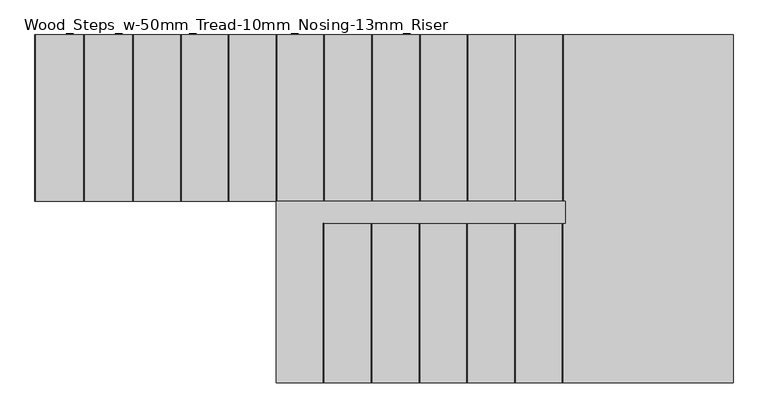
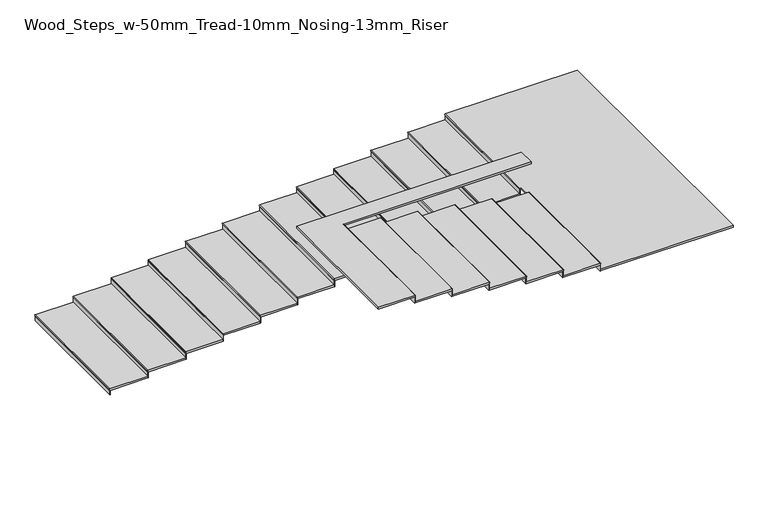
"""IFC4 building model written with IfcOpenShell, lengths in millimetres: stair flight geometry, Wood_Steps_w-50mm_Tread-10mm_Nosing-13mm_Riser."""

from ifc_helpers import new_model, si_unit, frame, origin, place, context, project, spatial, circle_curve, faceted_brep, source, transform, mapped, element, save
from ifc_brep_helpers import plane_surface, cylinder_surface, advanced_brep


def wood_steps_w_50mm_tread_10mm_nosing_13mm_riser_e98e060e(model_context):
    return source(origin(), model_context, "Body", "SolidModel", [
        advanced_brep(
        [(-49046.7440401, 412.2005214, 146.6666667), (-49046.7440401, 412.2005214, 166.6666667), (-49046.7440401, 3859.4375818, 166.6666667), (-49046.7440401, 3859.4375818, 146.6666667), (-48030.7440401, 3859.4375818, 166.6666667), (-48030.7440401, 412.2005214, 166.6666667), (-49046.7440401, 3859.4375818, 116.6666667), (-48030.7440401, 3859.4375818, 116.6666667), (-48030.7440401, 412.2005214, 116.6666667), (-49046.7440401, 412.2005214, 116.6666667)],
        [
            (0, 1, circle_curve(frame((-49046.7440401, 412.2005214, 156.6666667), z_axis=(0.0, 1.0, 0.0), x_axis=(1.0, 0.0, 0.0)), 10.0)),
            (1, 2),
            (2, 3, circle_curve(frame((-49046.7440401, 3859.4375818, 156.6666667), z_axis=(0.0, -1.0, 0.0), x_axis=(1.0, 0.0, 0.0)), 10.0)),
            (3, 0),
            (4, 2),
            (1, 5),
            (5, 4),
            (6, 7),
            (7, 8),
            (8, 9),
            (9, 6),
            (4, 7),
            (6, 3),
            (9, 0),
            (8, 5),
        ],
        [
            cylinder_surface(frame((-49046.7440401, 412.2005214, 156.6666667), z_axis=(0.0, -1.0, 0.0), x_axis=(1.0, 0.0, 0.0)), 10.0),
            plane_surface(frame((-49056.7440401, 3859.4375818, 166.6666667), z_axis=(0.0, 0.0, 1.0), x_axis=(-1.0, 0.0, 0.0))),
            plane_surface(frame((-49056.7440401, 3859.4375818, 116.6666667), z_axis=(0.0, 0.0, -1.0), x_axis=(1.0, 0.0, 0.0))),
            plane_surface(frame((-48030.7440401, 3859.4375818, 166.6666667), z_axis=(0.0, 1.0, 0.0), x_axis=(0.0, 0.0, -1.0))),
            plane_surface(frame((-49046.7440401, 3859.4375818, 166.6666667), z_axis=(-1.0, 0.0, 0.0), x_axis=(0.0, 0.0, -1.0))),
            plane_surface(frame((-49046.7440401, 412.2005214, 166.6666667), z_axis=(0.0, -1.0, 0.0), x_axis=(0.0, 0.0, -1.0))),
            plane_surface(frame((-48030.7440401, 412.2005214, 166.6666667), z_axis=(1.0, 0.0, 0.0), x_axis=(0.0, 0.0, -1.0))),
        ],
        [
            (0, [[1, 2, 3, 4]]),
            (1, [[5, -2, 6, 7]]),
            (2, [[8, 9, 10, 11]]),
            (3, [[-5, 12, -8, 13, -3]]),
            (4, [[-11, 14, -4, -13]]),
            (5, [[-6, -1, -14, -10, 15]]),
            (6, [[-7, -15, -9, -12]]),
        ],
    ),
        faceted_brep([(-49046.7440401, 412.2005214, 116.6666667), (-49046.7440401, 412.2005214, 0.0), (-49034.2440401, 412.2005214, 0.0), (-49034.2440401, 412.2005214, 116.6666667), (-49046.7440401, 3859.4375818, 116.6666667), (-49034.2440401, 3859.4375818, 116.6666667), (-49034.2440401, 3859.4375818, 0.0), (-49046.7440401, 3859.4375818, 0.0)], [[[0, 1, 2, 3]], [[4, 5, 6, 7]], [[1, 0, 4, 7]], [[2, 1, 7, 6]], [[3, 2, 6, 5]], [[0, 3, 5, 4]]]),
        faceted_brep([(-48030.7440401, 412.2005214, 283.3333333), (-48030.7440401, 412.2005214, 116.6666667), (-48018.2440401, 412.2005214, 116.6666667), (-48018.2440401, 412.2005214, 283.3333333), (-48030.7440401, 3859.4375818, 283.3333333), (-48018.2440401, 3859.4375818, 283.3333333), (-48018.2440401, 3859.4375818, 116.6666667), (-48030.7440401, 3859.4375818, 116.6666667)], [[[0, 1, 2, 3]], [[4, 5, 6, 7]], [[1, 0, 4, 7]], [[2, 1, 7, 6]], [[3, 2, 6, 5]], [[0, 3, 5, 4]]]),
        advanced_brep(
        [(-47014.7440401, 3859.4375818, 333.3333333), (-48030.7440401, 3859.4375818, 333.3333333), (-48030.7440401, 412.2005214, 333.3333333), (-47014.7440401, 412.2005214, 333.3333333), (-48030.7440401, 3859.4375818, 283.3333333), (-47014.7440401, 3859.4375818, 283.3333333), (-47014.7440401, 412.2005214, 283.3333333), (-48030.7440401, 412.2005214, 283.3333333), (-48030.7440401, 3859.4375818, 313.3333333), (-48030.7440401, 412.2005214, 313.3333333)],
        [
            (0, 1),
            (1, 2),
            (2, 3),
            (3, 0),
            (4, 5),
            (5, 6),
            (6, 7),
            (7, 4),
            (0, 5),
            (4, 8),
            (8, 1, circle_curve(frame((-48030.7440401, 3859.4375818, 323.3333333), z_axis=(0.0, 1.0, 0.0), x_axis=(1.0, 0.0, 0.0)), 10.0)),
            (7, 9),
            (9, 8),
            (2, 9, circle_curve(frame((-48030.7440401, 412.2005214, 323.3333333), z_axis=(0.0, -1.0, 0.0), x_axis=(1.0, 0.0, 0.0)), 10.0)),
            (6, 3),
        ],
        [
            plane_surface(frame((-49056.7440401, 3859.4375818, 333.3333333), z_axis=(0.0, 0.0, 1.0), x_axis=(-1.0, 0.0, 0.0))),
            plane_surface(frame((-49056.7440401, 3859.4375818, 283.3333333), z_axis=(0.0, 0.0, -1.0), x_axis=(1.0, 0.0, 0.0))),
            plane_surface(frame((-47014.7440401, 3859.4375818, 333.3333333), z_axis=(0.0, 1.0, 0.0), x_axis=(0.0, 0.0, -1.0))),
            plane_surface(frame((-48030.7440401, 3859.4375818, 333.3333333), z_axis=(-1.0, 0.0, 0.0), x_axis=(0.0, 0.0, -1.0))),
            plane_surface(frame((-48030.7440401, 412.2005214, 333.3333333), z_axis=(0.0, -1.0, 0.0), x_axis=(0.0, 0.0, -1.0))),
            plane_surface(frame((-47014.7440401, 412.2005214, 333.3333333), z_axis=(1.0, 0.0, 0.0), x_axis=(0.0, 0.0, -1.0))),
            cylinder_surface(frame((-48030.7440401, 412.2005214, 323.3333333), z_axis=(0.0, -1.0, 0.0), x_axis=(1.0, 0.0, 0.0)), 10.0),
        ],
        [
            (0, [[1, 2, 3, 4]]),
            (1, [[5, 6, 7, 8]]),
            (2, [[-1, 9, -5, 10, 11]]),
            (3, [[-8, 12, 13, -10]]),
            (4, [[-3, 14, -12, -7, 15]]),
            (5, [[-4, -15, -6, -9]]),
            (6, [[-14, -2, -11, -13]]),
        ],
    ),
        faceted_brep([(-47014.7440401, 412.2005214, 450.0), (-47014.7440401, 412.2005214, 283.3333333), (-47002.2440401, 412.2005214, 283.3333333), (-47002.2440401, 412.2005214, 450.0), (-47014.7440401, 3859.4375818, 450.0), (-47002.2440401, 3859.4375818, 450.0), (-47002.2440401, 3859.4375818, 283.3333333), (-47014.7440401, 3859.4375818, 283.3333333)], [[[0, 1, 2, 3]], [[4, 5, 6, 7]], [[1, 0, 4, 7]], [[2, 1, 7, 6]], [[3, 2, 6, 5]], [[0, 3, 5, 4]]]),
        advanced_brep(
        [(-46024.1440401, 3859.4375818, 500.0), (-47014.7440401, 3859.4375818, 500.0), (-47014.7440401, 412.2005214, 500.0), (-46024.1440401, 412.2005214, 500.0), (-47014.7440401, 3859.4375818, 450.0), (-46024.1440401, 3859.4375818, 450.0), (-46024.1440401, 412.2005214, 450.0), (-47014.7440401, 412.2005214, 450.0), (-47014.7440401, 3859.4375818, 480.0), (-47014.7440401, 412.2005214, 480.0)],
        [
            (0, 1),
            (1, 2),
            (2, 3),
            (3, 0),
            (4, 5),
            (5, 6),
            (6, 7),
            (7, 4),
            (0, 5),
            (4, 8),
            (8, 1, circle_curve(frame((-47014.7440401, 3859.4375818, 490.0), z_axis=(0.0, 1.0, 0.0), x_axis=(1.0, 0.0, 0.0)), 10.0)),
            (7, 9),
            (9, 8),
            (2, 9, circle_curve(frame((-47014.7440401, 412.2005214, 490.0), z_axis=(0.0, -1.0, 0.0), x_axis=(1.0, 0.0, 0.0)), 10.0)),
            (6, 3),
        ],
        [
            plane_surface(frame((-49056.7440401, 3859.4375818, 500.0), z_axis=(0.0, 0.0, 1.0), x_axis=(-1.0, 0.0, 0.0))),
            plane_surface(frame((-49056.7440401, 3859.4375818, 450.0), z_axis=(0.0, 0.0, -1.0), x_axis=(1.0, 0.0, 0.0))),
            plane_surface(frame((-46024.1440401, 3859.4375818, 500.0), z_axis=(0.0, 1.0, 0.0), x_axis=(0.0, 0.0, -1.0))),
            plane_surface(frame((-47014.7440401, 3859.4375818, 500.0), z_axis=(-1.0, 0.0, 0.0), x_axis=(0.0, 0.0, -1.0))),
            plane_surface(frame((-47014.7440401, 412.2005214, 500.0), z_axis=(0.0, -1.0, 0.0), x_axis=(0.0, 0.0, -1.0))),
            plane_surface(frame((-46024.1440401, 412.2005214, 500.0), z_axis=(1.0, 0.0, 0.0), x_axis=(0.0, 0.0, -1.0))),
            cylinder_surface(frame((-47014.7440401, 412.2005214, 490.0), z_axis=(0.0, -1.0, 0.0), x_axis=(1.0, 0.0, 0.0)), 10.0),
        ],
        [
            (0, [[1, 2, 3, 4]]),
            (1, [[5, 6, 7, 8]]),
            (2, [[-1, 9, -5, 10, 11]]),
            (3, [[-8, 12, 13, -10]]),
            (4, [[-3, 14, -12, -7, 15]]),
            (5, [[-4, -15, -6, -9]]),
            (6, [[-14, -2, -11, -13]]),
        ],
    ),
        faceted_brep([(-46024.1440401, 412.2005214, 616.6666667), (-46024.1440401, 412.2005214, 450.0), (-46011.6440401, 412.2005214, 450.0), (-46011.6440401, 412.2005214, 616.6666667), (-46024.1440401, 3859.4375818, 616.6666667), (-46011.6440401, 3859.4375818, 616.6666667), (-46011.6440401, 3859.4375818, 450.0), (-46024.1440401, 3859.4375818, 450.0)], [[[0, 1, 2, 3]], [[4, 5, 6, 7]], [[1, 0, 4, 7]], [[2, 1, 7, 6]], [[3, 2, 6, 5]], [[0, 3, 5, 4]]]),
        advanced_brep(
        [(-45033.5440401, 3859.4375818, 666.6666667), (-46024.1440401, 3859.4375818, 666.6666667), (-46024.1440401, 412.2005214, 666.6666667), (-45033.5440401, 412.2005214, 666.6666667), (-46024.1440401, 3859.4375818, 616.6666667), (-45033.5440401, 3859.4375818, 616.6666667), (-45033.5440401, 412.2005214, 616.6666667), (-46024.1440401, 412.2005214, 616.6666667), (-46024.1440401, 3859.4375818, 646.6666667), (-46024.1440401, 412.2005214, 646.6666667)],
        [
            (0, 1),
            (1, 2),
            (2, 3),
            (3, 0),
            (4, 5),
            (5, 6),
            (6, 7),
            (7, 4),
            (0, 5),
            (4, 8),
            (8, 1, circle_curve(frame((-46024.1440401, 3859.4375818, 656.6666667), z_axis=(0.0, 1.0, 0.0), x_axis=(1.0, 0.0, 0.0)), 10.0)),
            (7, 9),
            (9, 8),
            (2, 9, circle_curve(frame((-46024.1440401, 412.2005214, 656.6666667), z_axis=(0.0, -1.0, 0.0), x_axis=(1.0, 0.0, 0.0)), 10.0)),
            (6, 3),
        ],
        [
            plane_surface(frame((-48066.1440401, 3859.4375818, 666.6666667), z_axis=(0.0, 0.0, 1.0), x_axis=(-1.0, 0.0, 0.0))),
            plane_surface(frame((-48066.1440401, 3859.4375818, 616.6666667), z_axis=(0.0, 0.0, -1.0), x_axis=(1.0, 0.0, 0.0))),
            plane_surface(frame((-45033.5440401, 3859.4375818, 666.6666667), z_axis=(0.0, 1.0, 0.0), x_axis=(0.0, 0.0, -1.0))),
            plane_surface(frame((-46024.1440401, 3859.4375818, 666.6666667), z_axis=(-1.0, 0.0, 0.0), x_axis=(0.0, 0.0, -1.0))),
            plane_surface(frame((-46024.1440401, 412.2005214, 666.6666667), z_axis=(0.0, -1.0, 0.0), x_axis=(0.0, 0.0, -1.0))),
            plane_surface(frame((-45033.5440401, 412.2005214, 666.6666667), z_axis=(1.0, 0.0, 0.0), x_axis=(0.0, 0.0, -1.0))),
            cylinder_surface(frame((-46024.1440401, 412.2005214, 656.6666667), z_axis=(0.0, -1.0, 0.0), x_axis=(1.0, 0.0, 0.0)), 10.0),
        ],
        [
            (0, [[1, 2, 3, 4]]),
            (1, [[5, 6, 7, 8]]),
            (2, [[-1, 9, -5, 10, 11]]),
            (3, [[-8, 12, 13, -10]]),
            (4, [[-3, 14, -12, -7, 15]]),
            (5, [[-4, -15, -6, -9]]),
            (6, [[-14, -2, -11, -13]]),
        ],
    ),
        faceted_brep([(-45033.5440401, 412.2005214, 783.3333333), (-45033.5440401, 412.2005214, 616.6666667), (-45021.0440401, 412.2005214, 616.6666667), (-45021.0440401, 412.2005214, 783.3333333), (-45033.5440401, 3859.4375818, 783.3333333), (-45021.0440401, 3859.4375818, 783.3333333), (-45021.0440401, 3859.4375818, 616.6666667), (-45033.5440401, 3859.4375818, 616.6666667)], [[[0, 1, 2, 3]], [[4, 5, 6, 7]], [[1, 0, 4, 7]], [[2, 1, 7, 6]], [[3, 2, 6, 5]], [[0, 3, 5, 4]]]),
        advanced_brep(
        [(-44042.9440401, 3859.4375818, 833.3333333), (-45033.5440401, 3859.4375818, 833.3333333), (-45033.5440401, 412.2005214, 833.3333333), (-44042.9440401, 412.2005214, 833.3333333), (-45033.5440401, 3859.4375818, 783.3333333), (-44042.9440401, 3859.4375818, 783.3333333), (-44042.9440401, 412.2005214, 783.3333333), (-45033.5440401, 412.2005214, 783.3333333), (-45033.5440401, 3859.4375818, 813.3333333), (-45033.5440401, 412.2005214, 813.3333333)],
        [
            (0, 1),
            (1, 2),
            (2, 3),
            (3, 0),
            (4, 5),
            (5, 6),
            (6, 7),
            (7, 4),
            (0, 5),
            (4, 8),
            (8, 1, circle_curve(frame((-45033.5440401, 3859.4375818, 823.3333333), z_axis=(0.0, 1.0, 0.0), x_axis=(1.0, 0.0, 0.0)), 10.0)),
            (7, 9),
            (9, 8),
            (2, 9, circle_curve(frame((-45033.5440401, 412.2005214, 823.3333333), z_axis=(0.0, -1.0, 0.0), x_axis=(1.0, 0.0, 0.0)), 10.0)),
            (6, 3),
        ],
        [
            plane_surface(frame((-47075.5440401, 3859.4375818, 833.3333333), z_axis=(0.0, 0.0, 1.0), x_axis=(-1.0, 0.0, 0.0))),
            plane_surface(frame((-47075.5440401, 3859.4375818, 783.3333333), z_axis=(0.0, 0.0, -1.0), x_axis=(1.0, 0.0, 0.0))),
            plane_surface(frame((-44042.9440401, 3859.4375818, 833.3333333), z_axis=(0.0, 1.0, 0.0), x_axis=(0.0, 0.0, -1.0))),
            plane_surface(frame((-45033.5440401, 3859.4375818, 833.3333333), z_axis=(-1.0, 0.0, 0.0), x_axis=(0.0, 0.0, -1.0))),
            plane_surface(frame((-45033.5440401, 412.2005214, 833.3333333), z_axis=(0.0, -1.0, 0.0), x_axis=(0.0, 0.0, -1.0))),
            plane_surface(frame((-44042.9440401, 412.2005214, 833.3333333), z_axis=(1.0, 0.0, 0.0), x_axis=(0.0, 0.0, -1.0))),
            cylinder_surface(frame((-45033.5440401, 412.2005214, 823.3333333), z_axis=(0.0, -1.0, 0.0), x_axis=(1.0, 0.0, 0.0)), 10.0),
        ],
        [
            (0, [[1, 2, 3, 4]]),
            (1, [[5, 6, 7, 8]]),
            (2, [[-1, 9, -5, 10, 11]]),
            (3, [[-8, 12, 13, -10]]),
            (4, [[-3, 14, -12, -7, 15]]),
            (5, [[-4, -15, -6, -9]]),
            (6, [[-14, -2, -11, -13]]),
        ],
    ),
        faceted_brep([(-44042.9440401, 412.2005214, 950.0), (-44042.9440401, 412.2005214, 783.3333333), (-44030.4440401, 412.2005214, 783.3333333), (-44030.4440401, 412.2005214, 950.0), (-44042.9440401, 3859.4375818, 950.0), (-44030.4440401, 3859.4375818, 950.0), (-44030.4440401, 3859.4375818, 783.3333333), (-44042.9440401, 3859.4375818, 783.3333333)], [[[0, 1, 2, 3]], [[4, 5, 6, 7]], [[1, 0, 4, 7]], [[2, 1, 7, 6]], [[3, 2, 6, 5]], [[0, 3, 5, 4]]]),
        advanced_brep(
        [(-43052.3440401, 3859.4375818, 1000.0), (-44042.9440401, 3859.4375818, 1000.0), (-44042.9440401, 412.2005214, 1000.0), (-43052.3440401, 412.2005214, 1000.0), (-44042.9440401, 3859.4375818, 950.0), (-43052.3440401, 3859.4375818, 950.0), (-43052.3440401, 412.2005214, 950.0), (-44042.9440401, 412.2005214, 950.0), (-44042.9440401, 3859.4375818, 980.0), (-44042.9440401, 412.2005214, 980.0)],
        [
            (0, 1),
            (1, 2),
            (2, 3),
            (3, 0),
            (4, 5),
            (5, 6),
            (6, 7),
            (7, 4),
            (0, 5),
            (4, 8),
            (8, 1, circle_curve(frame((-44042.9440401, 3859.4375818, 990.0), z_axis=(0.0, 1.0, 0.0), x_axis=(1.0, 0.0, 0.0)), 10.0)),
            (7, 9),
            (9, 8),
            (2, 9, circle_curve(frame((-44042.9440401, 412.2005214, 990.0), z_axis=(0.0, -1.0, 0.0), x_axis=(1.0, 0.0, 0.0)), 10.0)),
            (6, 3),
        ],
        [
            plane_surface(frame((-46084.9440401, 3859.4375818, 1000.0), z_axis=(0.0, 0.0, 1.0), x_axis=(-1.0, 0.0, 0.0))),
            plane_surface(frame((-46084.9440401, 3859.4375818, 950.0), z_axis=(0.0, 0.0, -1.0), x_axis=(1.0, 0.0, 0.0))),
            plane_surface(frame((-43052.3440401, 3859.4375818, 1000.0), z_axis=(0.0, 1.0, 0.0), x_axis=(0.0, 0.0, -1.0))),
            plane_surface(frame((-44042.9440401, 3859.4375818, 1000.0), z_axis=(-1.0, 0.0, 0.0), x_axis=(0.0, 0.0, -1.0))),
            plane_surface(frame((-44042.9440401, 412.2005214, 1000.0), z_axis=(0.0, -1.0, 0.0), x_axis=(0.0, 0.0, -1.0))),
            plane_surface(frame((-43052.3440401, 412.2005214, 1000.0), z_axis=(1.0, 0.0, 0.0), x_axis=(0.0, 0.0, -1.0))),
            cylinder_surface(frame((-44042.9440401, 412.2005214, 990.0), z_axis=(0.0, -1.0, 0.0), x_axis=(1.0, 0.0, 0.0)), 10.0),
        ],
        [
            (0, [[1, 2, 3, 4]]),
            (1, [[5, 6, 7, 8]]),
            (2, [[-1, 9, -5, 10, 11]]),
            (3, [[-8, 12, 13, -10]]),
            (4, [[-3, 14, -12, -7, 15]]),
            (5, [[-4, -15, -6, -9]]),
            (6, [[-14, -2, -11, -13]]),
        ],
    ),
        faceted_brep([(-43052.3440401, 412.2005214, 1116.6666667), (-43052.3440401, 412.2005214, 950.0), (-43039.8440401, 412.2005214, 950.0), (-43039.8440401, 412.2005214, 1116.6666667), (-43052.3440401, 3859.4375818, 1116.6666667), (-43039.8440401, 3859.4375818, 1116.6666667), (-43039.8440401, 3859.4375818, 950.0), (-43052.3440401, 3859.4375818, 950.0)], [[[0, 1, 2, 3]], [[4, 5, 6, 7]], [[1, 0, 4, 7]], [[2, 1, 7, 6]], [[3, 2, 6, 5]], [[0, 3, 5, 4]]]),
        advanced_brep(
        [(-42061.7440401, 3859.4375818, 1166.6666667), (-43052.3440401, 3859.4375818, 1166.6666667), (-43052.3440401, 412.2005214, 1166.6666667), (-42061.7440401, 412.2005214, 1166.6666667), (-43052.3440401, 3859.4375818, 1116.6666667), (-42061.7440401, 3859.4375818, 1116.6666667), (-42061.7440401, 412.2005214, 1116.6666667), (-43052.3440401, 412.2005214, 1116.6666667), (-43052.3440401, 3859.4375818, 1146.6666667), (-43052.3440401, 412.2005214, 1146.6666667)],
        [
            (0, 1),
            (1, 2),
            (2, 3),
            (3, 0),
            (4, 5),
            (5, 6),
            (6, 7),
            (7, 4),
            (0, 5),
            (4, 8),
            (8, 1, circle_curve(frame((-43052.3440401, 3859.4375818, 1156.6666667), z_axis=(0.0, 1.0, 0.0), x_axis=(1.0, 0.0, 0.0)), 10.0)),
            (7, 9),
            (9, 8),
            (2, 9, circle_curve(frame((-43052.3440401, 412.2005214, 1156.6666667), z_axis=(0.0, -1.0, 0.0), x_axis=(1.0, 0.0, 0.0)), 10.0)),
            (6, 3),
        ],
        [
            plane_surface(frame((-45094.3440401, 3859.4375818, 1166.6666667), z_axis=(0.0, 0.0, 1.0), x_axis=(-1.0, 0.0, 0.0))),
            plane_surface(frame((-45094.3440401, 3859.4375818, 1116.6666667), z_axis=(0.0, 0.0, -1.0), x_axis=(1.0, 0.0, 0.0))),
            plane_surface(frame((-42061.7440401, 3859.4375818, 1166.6666667), z_axis=(0.0, 1.0, 0.0), x_axis=(0.0, 0.0, -1.0))),
            plane_surface(frame((-43052.3440401, 3859.4375818, 1166.6666667), z_axis=(-1.0, 0.0, 0.0), x_axis=(0.0, 0.0, -1.0))),
            plane_surface(frame((-43052.3440401, 412.2005214, 1166.6666667), z_axis=(0.0, -1.0, 0.0), x_axis=(0.0, 0.0, -1.0))),
            plane_surface(frame((-42061.7440401, 412.2005214, 1166.6666667), z_axis=(1.0, 0.0, 0.0), x_axis=(0.0, 0.0, -1.0))),
            cylinder_surface(frame((-43052.3440401, 412.2005214, 1156.6666667), z_axis=(0.0, -1.0, 0.0), x_axis=(1.0, 0.0, 0.0)), 10.0),
        ],
        [
            (0, [[1, 2, 3, 4]]),
            (1, [[5, 6, 7, 8]]),
            (2, [[-1, 9, -5, 10, 11]]),
            (3, [[-8, 12, 13, -10]]),
            (4, [[-3, 14, -12, -7, 15]]),
            (5, [[-4, -15, -6, -9]]),
            (6, [[-14, -2, -11, -13]]),
        ],
    ),
        faceted_brep([(-42061.7440401, 412.2005214, 1283.3333333), (-42061.7440401, 412.2005214, 1116.6666667), (-42049.2440401, 412.2005214, 1116.6666667), (-42049.2440401, 412.2005214, 1283.3333333), (-42061.7440401, 3859.4375818, 1283.3333333), (-42049.2440401, 3859.4375818, 1283.3333333), (-42049.2440401, 3859.4375818, 1116.6666667), (-42061.7440401, 3859.4375818, 1116.6666667)], [[[0, 1, 2, 3]], [[4, 5, 6, 7]], [[1, 0, 4, 7]], [[2, 1, 7, 6]], [[3, 2, 6, 5]], [[0, 3, 5, 4]]]),
        advanced_brep(
        [(-41071.1440401, 3859.4375818, 1333.3333333), (-42061.7440401, 3859.4375818, 1333.3333333), (-42061.7440401, 412.2005214, 1333.3333333), (-41071.1440401, 412.2005214, 1333.3333333), (-42061.7440401, 3859.4375818, 1283.3333333), (-41071.1440401, 3859.4375818, 1283.3333333), (-41071.1440401, 412.2005214, 1283.3333333), (-42061.7440401, 412.2005214, 1283.3333333), (-42061.7440401, 3859.4375818, 1313.3333333), (-42061.7440401, 412.2005214, 1313.3333333)],
        [
            (0, 1),
            (1, 2),
            (2, 3),
            (3, 0),
            (4, 5),
            (5, 6),
            (6, 7),
            (7, 4),
            (0, 5),
            (4, 8),
            (8, 1, circle_curve(frame((-42061.7440401, 3859.4375818, 1323.3333333), z_axis=(0.0, 1.0, 0.0), x_axis=(1.0, 0.0, 0.0)), 10.0)),
            (7, 9),
            (9, 8),
            (2, 9, circle_curve(frame((-42061.7440401, 412.2005214, 1323.3333333), z_axis=(0.0, -1.0, 0.0), x_axis=(1.0, 0.0, 0.0)), 10.0)),
            (6, 3),
        ],
        [
            plane_surface(frame((-44103.7440401, 3859.4375818, 1333.3333333), z_axis=(0.0, 0.0, 1.0), x_axis=(-1.0, 0.0, 0.0))),
            plane_surface(frame((-44103.7440401, 3859.4375818, 1283.3333333), z_axis=(0.0, 0.0, -1.0), x_axis=(1.0, 0.0, 0.0))),
            plane_surface(frame((-41071.1440401, 3859.4375818, 1333.3333333), z_axis=(0.0, 1.0, 0.0), x_axis=(0.0, 0.0, -1.0))),
            plane_surface(frame((-42061.7440401, 3859.4375818, 1333.3333333), z_axis=(-1.0, 0.0, 0.0), x_axis=(0.0, 0.0, -1.0))),
            plane_surface(frame((-42061.7440401, 412.2005214, 1333.3333333), z_axis=(0.0, -1.0, 0.0), x_axis=(0.0, 0.0, -1.0))),
            plane_surface(frame((-41071.1440401, 412.2005214, 1333.3333333), z_axis=(1.0, 0.0, 0.0), x_axis=(0.0, 0.0, -1.0))),
            cylinder_surface(frame((-42061.7440401, 412.2005214, 1323.3333333), z_axis=(0.0, -1.0, 0.0), x_axis=(1.0, 0.0, 0.0)), 10.0),
        ],
        [
            (0, [[1, 2, 3, 4]]),
            (1, [[5, 6, 7, 8]]),
            (2, [[-1, 9, -5, 10, 11]]),
            (3, [[-8, 12, 13, -10]]),
            (4, [[-3, 14, -12, -7, 15]]),
            (5, [[-4, -15, -6, -9]]),
            (6, [[-14, -2, -11, -13]]),
        ],
    ),
        faceted_brep([(-41071.1440401, 412.2005214, 1450.0), (-41071.1440401, 412.2005214, 1283.3333333), (-41058.6440401, 412.2005214, 1283.3333333), (-41058.6440401, 412.2005214, 1450.0), (-41071.1440401, 3859.4375818, 1450.0), (-41058.6440401, 3859.4375818, 1450.0), (-41058.6440401, 3859.4375818, 1283.3333333), (-41071.1440401, 3859.4375818, 1283.3333333)], [[[0, 1, 2, 3]], [[4, 5, 6, 7]], [[1, 0, 4, 7]], [[2, 1, 7, 6]], [[3, 2, 6, 5]], [[0, 3, 5, 4]]]),
        advanced_brep(
        [(-40080.5440401, 3859.4375818, 1500.0), (-41071.1440401, 3859.4375818, 1500.0), (-41071.1440401, 412.2005214, 1500.0), (-40080.5440401, 412.2005214, 1500.0), (-41071.1440401, 3859.4375818, 1450.0), (-40080.5440401, 3859.4375818, 1450.0), (-40080.5440401, 412.2005214, 1450.0), (-41071.1440401, 412.2005214, 1450.0), (-41071.1440401, 3859.4375818, 1480.0), (-41071.1440401, 412.2005214, 1480.0)],
        [
            (0, 1),
            (1, 2),
            (2, 3),
            (3, 0),
            (4, 5),
            (5, 6),
            (6, 7),
            (7, 4),
            (0, 5),
            (4, 8),
            (8, 1, circle_curve(frame((-41071.1440401, 3859.4375818, 1490.0), z_axis=(0.0, 1.0, 0.0), x_axis=(1.0, 0.0, 0.0)), 10.0)),
            (7, 9),
            (9, 8),
            (2, 9, circle_curve(frame((-41071.1440401, 412.2005214, 1490.0), z_axis=(0.0, -1.0, 0.0), x_axis=(1.0, 0.0, 0.0)), 10.0)),
            (6, 3),
        ],
        [
            plane_surface(frame((-43113.1440401, 3859.4375818, 1500.0), z_axis=(0.0, 0.0, 1.0), x_axis=(-1.0, 0.0, 0.0))),
            plane_surface(frame((-43113.1440401, 3859.4375818, 1450.0), z_axis=(0.0, 0.0, -1.0), x_axis=(1.0, 0.0, 0.0))),
            plane_surface(frame((-40080.5440401, 3859.4375818, 1500.0), z_axis=(0.0, 1.0, 0.0), x_axis=(0.0, 0.0, -1.0))),
            plane_surface(frame((-41071.1440401, 3859.4375818, 1500.0), z_axis=(-1.0, 0.0, 0.0), x_axis=(0.0, 0.0, -1.0))),
            plane_surface(frame((-41071.1440401, 412.2005214, 1500.0), z_axis=(0.0, -1.0, 0.0), x_axis=(0.0, 0.0, -1.0))),
            plane_surface(frame((-40080.5440401, 412.2005214, 1500.0), z_axis=(1.0, 0.0, 0.0), x_axis=(0.0, 0.0, -1.0))),
            cylinder_surface(frame((-41071.1440401, 412.2005214, 1490.0), z_axis=(0.0, -1.0, 0.0), x_axis=(1.0, 0.0, 0.0)), 10.0),
        ],
        [
            (0, [[1, 2, 3, 4]]),
            (1, [[5, 6, 7, 8]]),
            (2, [[-1, 9, -5, 10, 11]]),
            (3, [[-8, 12, 13, -10]]),
            (4, [[-3, 14, -12, -7, 15]]),
            (5, [[-4, -15, -6, -9]]),
            (6, [[-14, -2, -11, -13]]),
        ],
    ),
        faceted_brep([(-40080.5440401, 412.2005214, 1616.6666667), (-40080.5440401, 412.2005214, 1450.0), (-40068.0440401, 412.2005214, 1450.0), (-40068.0440401, 412.2005214, 1616.6666667), (-40080.5440401, 3859.4375818, 1616.6666667), (-40068.0440401, 3859.4375818, 1616.6666667), (-40068.0440401, 3859.4375818, 1450.0), (-40080.5440401, 3859.4375818, 1450.0)], [[[0, 1, 2, 3]], [[4, 5, 6, 7]], [[1, 0, 4, 7]], [[2, 1, 7, 6]], [[3, 2, 6, 5]], [[0, 3, 5, 4]]]),
        advanced_brep(
        [(-39089.9440401, 3859.4375818, 1666.6666667), (-40080.5440401, 3859.4375818, 1666.6666667), (-40080.5440401, 412.2005214, 1666.6666667), (-39089.9440401, 412.2005214, 1666.6666667), (-40080.5440401, 3859.4375818, 1616.6666667), (-39089.9440401, 3859.4375818, 1616.6666667), (-39089.9440401, 412.2005214, 1616.6666667), (-40080.5440401, 412.2005214, 1616.6666667), (-40080.5440401, 3859.4375818, 1646.6666667), (-40080.5440401, 412.2005214, 1646.6666667)],
        [
            (0, 1),
            (1, 2),
            (2, 3),
            (3, 0),
            (4, 5),
            (5, 6),
            (6, 7),
            (7, 4),
            (0, 5),
            (4, 8),
            (8, 1, circle_curve(frame((-40080.5440401, 3859.4375818, 1656.6666667), z_axis=(0.0, 1.0, 0.0), x_axis=(1.0, 0.0, 0.0)), 10.0)),
            (7, 9),
            (9, 8),
            (2, 9, circle_curve(frame((-40080.5440401, 412.2005214, 1656.6666667), z_axis=(0.0, -1.0, 0.0), x_axis=(1.0, 0.0, 0.0)), 10.0)),
            (6, 3),
        ],
        [
            plane_surface(frame((-42122.5440401, 3859.4375818, 1666.6666667), z_axis=(0.0, 0.0, 1.0), x_axis=(-1.0, 0.0, 0.0))),
            plane_surface(frame((-42122.5440401, 3859.4375818, 1616.6666667), z_axis=(0.0, 0.0, -1.0), x_axis=(1.0, 0.0, 0.0))),
            plane_surface(frame((-39089.9440401, 3859.4375818, 1666.6666667), z_axis=(0.0, 1.0, 0.0), x_axis=(0.0, 0.0, -1.0))),
            plane_surface(frame((-40080.5440401, 3859.4375818, 1666.6666667), z_axis=(-1.0, 0.0, 0.0), x_axis=(0.0, 0.0, -1.0))),
            plane_surface(frame((-40080.5440401, 412.2005214, 1666.6666667), z_axis=(0.0, -1.0, 0.0), x_axis=(0.0, 0.0, -1.0))),
            plane_surface(frame((-39089.9440401, 412.2005214, 1666.6666667), z_axis=(1.0, 0.0, 0.0), x_axis=(0.0, 0.0, -1.0))),
            cylinder_surface(frame((-40080.5440401, 412.2005214, 1656.6666667), z_axis=(0.0, -1.0, 0.0), x_axis=(1.0, 0.0, 0.0)), 10.0),
        ],
        [
            (0, [[1, 2, 3, 4]]),
            (1, [[5, 6, 7, 8]]),
            (2, [[-1, 9, -5, 10, 11]]),
            (3, [[-8, 12, 13, -10]]),
            (4, [[-3, 14, -12, -7, 15]]),
            (5, [[-4, -15, -6, -9]]),
            (6, [[-14, -2, -11, -13]]),
        ],
    ),
        faceted_brep([(-39089.9440401, 412.2005214, 1783.3333333), (-39089.9440401, 412.2005214, 1616.6666667), (-39077.4440401, 412.2005214, 1616.6666667), (-39077.4440401, 412.2005214, 1783.3333333), (-39089.9440401, 3859.4375818, 1783.3333333), (-39077.4440401, 3859.4375818, 1783.3333333), (-39077.4440401, 3859.4375818, 1616.6666667), (-39089.9440401, 3859.4375818, 1616.6666667)], [[[0, 1, 2, 3]], [[4, 5, 6, 7]], [[1, 0, 4, 7]], [[2, 1, 7, 6]], [[3, 2, 6, 5]], [[0, 3, 5, 4]]]),
        advanced_brep(
        [(-38099.3440401, 3859.4375818, 1833.3333333), (-39089.9440401, 3859.4375818, 1833.3333333), (-39089.9440401, 412.2005214, 1833.3333333), (-38099.3440401, 412.2005214, 1833.3333333), (-39089.9440401, 3859.4375818, 1783.3333333), (-38099.3440401, 3859.4375818, 1783.3333333), (-38099.3440401, 412.2005214, 1783.3333333), (-39089.9440401, 412.2005214, 1783.3333333), (-39089.9440401, 3859.4375818, 1813.3333333), (-39089.9440401, 412.2005214, 1813.3333333)],
        [
            (0, 1),
            (1, 2),
            (2, 3),
            (3, 0),
            (4, 5),
            (5, 6),
            (6, 7),
            (7, 4),
            (0, 5),
            (4, 8),
            (8, 1, circle_curve(frame((-39089.9440401, 3859.4375818, 1823.3333333), z_axis=(0.0, 1.0, 0.0), x_axis=(1.0, 0.0, 0.0)), 10.0)),
            (7, 9),
            (9, 8),
            (2, 9, circle_curve(frame((-39089.9440401, 412.2005214, 1823.3333333), z_axis=(0.0, -1.0, 0.0), x_axis=(1.0, 0.0, 0.0)), 10.0)),
            (6, 3),
        ],
        [
            plane_surface(frame((-41131.9440401, 3859.4375818, 1833.3333333), z_axis=(0.0, 0.0, 1.0), x_axis=(-1.0, 0.0, 0.0))),
            plane_surface(frame((-41131.9440401, 3859.4375818, 1783.3333333), z_axis=(0.0, 0.0, -1.0), x_axis=(1.0, 0.0, 0.0))),
            plane_surface(frame((-38099.3440401, 3859.4375818, 1833.3333333), z_axis=(0.0, 1.0, 0.0), x_axis=(0.0, 0.0, -1.0))),
            plane_surface(frame((-39089.9440401, 3859.4375818, 1833.3333333), z_axis=(-1.0, 0.0, 0.0), x_axis=(0.0, 0.0, -1.0))),
            plane_surface(frame((-39089.9440401, 412.2005214, 1833.3333333), z_axis=(0.0, -1.0, 0.0), x_axis=(0.0, 0.0, -1.0))),
            plane_surface(frame((-38099.3440401, 412.2005214, 1833.3333333), z_axis=(1.0, 0.0, 0.0), x_axis=(0.0, 0.0, -1.0))),
            cylinder_surface(frame((-39089.9440401, 412.2005214, 1823.3333333), z_axis=(0.0, -1.0, 0.0), x_axis=(1.0, 0.0, 0.0)), 10.0),
        ],
        [
            (0, [[1, 2, 3, 4]]),
            (1, [[5, 6, 7, 8]]),
            (2, [[-1, 9, -5, 10, 11]]),
            (3, [[-8, 12, 13, -10]]),
            (4, [[-3, 14, -12, -7, 15]]),
            (5, [[-4, -15, -6, -9]]),
            (6, [[-14, -2, -11, -13]]),
        ],
    ),
        faceted_brep([(-38099.3440401, 412.2005214, 1950.0), (-38099.3440401, 412.2005214, 1783.3333333), (-38086.8440401, 412.2005214, 1783.3333333), (-38086.8440401, 412.2005214, 1950.0), (-38099.3440401, 3859.4375818, 1950.0), (-38086.8440401, 3859.4375818, 1950.0), (-38086.8440401, 3859.4375818, 1783.3333333), (-38099.3440401, 3859.4375818, 1783.3333333)], [[[0, 1, 2, 3]], [[4, 5, 6, 7]], [[1, 0, 4, 7]], [[2, 1, 7, 6]], [[3, 2, 6, 5]], [[0, 3, 5, 4]]]),
        advanced_brep(
        [(-38119.3440401, -3354.1624182, 2000.0), (-34578.7440401, -3354.1624182, 2000.0), (-34578.7440401, 3859.4375818, 2000.0), (-38099.3440401, 3859.4375818, 2000.0), (-38099.3440401, 412.2005214, 2000.0), (-38062.0088218, 412.2005214, 2000.0), (-38062.0088218, -44.9994786, 2000.0), (-38119.3440401, -44.9994786, 2000.0), (-34578.7440401, -3354.1624182, 1950.0), (-38119.3440401, -3354.1624182, 1950.0), (-38119.3440401, -44.9994786, 1950.0), (-38062.0088218, -44.9994786, 1950.0), (-38062.0088218, 412.2005214, 1950.0), (-38099.3440401, 412.2005214, 1950.0), (-38099.3440401, 3859.4375818, 1950.0), (-34578.7440401, 3859.4375818, 1950.0), (-38099.3440401, 3859.4375818, 1980.0), (-38099.3440401, 412.2005214, 1980.0)],
        [
            (0, 1),
            (1, 2),
            (2, 3),
            (3, 4),
            (4, 5),
            (5, 6),
            (6, 7),
            (7, 0),
            (8, 9),
            (9, 10),
            (10, 11),
            (11, 12),
            (12, 13),
            (13, 14),
            (14, 15),
            (15, 8),
            (0, 9),
            (8, 1),
            (15, 2),
            (14, 16),
            (16, 3, circle_curve(frame((-38099.3440401, 3859.4375818, 1990.0), z_axis=(0.0, 1.0, 0.0), x_axis=(1.0, 0.0, 0.0)), 10.0)),
            (13, 17),
            (17, 16),
            (4, 17, circle_curve(frame((-38099.3440401, 412.2005214, 1990.0), z_axis=(0.0, -1.0, 0.0), x_axis=(1.0, 0.0, 0.0)), 10.0)),
            (12, 5),
            (11, 6),
            (10, 7),
        ],
        [
            plane_surface(frame((-34578.7440401, -3354.1624182, 2000.0), z_axis=(0.0, 0.0, 1.0), x_axis=(1.0, 0.0, 0.0))),
            plane_surface(frame((-34578.7440401, -3354.1624182, 1950.0), z_axis=(0.0, 0.0, -1.0), x_axis=(-1.0, 0.0, 0.0))),
            plane_surface(frame((-38119.3440401, -3354.1624182, 2000.0), z_axis=(0.0, -1.0, 0.0), x_axis=(0.0, 0.0, -1.0))),
            plane_surface(frame((-34578.7440401, -3354.1624182, 2000.0), z_axis=(1.0, 0.0, 0.0), x_axis=(0.0, 0.0, -1.0))),
            plane_surface(frame((-34578.7440401, 3859.4375818, 2000.0), z_axis=(0.0, 1.0, 0.0), x_axis=(0.0, 0.0, -1.0))),
            plane_surface(frame((-38099.3440401, 3859.4375818, 2000.0), z_axis=(-1.0, 0.0, 0.0), x_axis=(0.0, 0.0, -1.0))),
            plane_surface(frame((-38099.3440401, 412.2005214, 2000.0), z_axis=(0.0, -1.0, 0.0), x_axis=(0.0, 0.0, -1.0))),
            plane_surface(frame((-38062.0088218, 412.2005214, 2000.0), z_axis=(-1.0, 0.0, 0.0), x_axis=(0.0, 0.0, -1.0))),
            plane_surface(frame((-38062.0088218, -44.9994786, 2000.0), z_axis=(0.0, 1.0, 0.0), x_axis=(0.0, 0.0, -1.0))),
            plane_surface(frame((-38119.3440401, -44.9994786, 2000.0), z_axis=(-1.0, 0.0, 0.0), x_axis=(0.0, 0.0, -1.0))),
            cylinder_surface(frame((-38099.3440401, 412.2005214, 1990.0), z_axis=(0.0, -1.0, 0.0), x_axis=(1.0, 0.0, 0.0)), 10.0),
        ],
        [
            (0, [[1, 2, 3, 4, 5, 6, 7, 8]]),
            (1, [[9, 10, 11, 12, 13, 14, 15, 16]]),
            (2, [[-1, 17, -9, 18]]),
            (3, [[-2, -18, -16, 19]]),
            (4, [[-3, -19, -15, 20, 21]]),
            (5, [[-14, 22, 23, -20]]),
            (6, [[-5, 24, -22, -13, 25]]),
            (7, [[-6, -25, -12, 26]]),
            (8, [[-7, -26, -11, 27]]),
            (9, [[-8, -27, -10, -17]]),
            (10, [[-24, -4, -21, -23]]),
        ],
    ),
        faceted_brep([(-38119.3440401, -44.9994786, 2116.6666667), (-38119.3440401, -44.9994786, 1950.0), (-38131.8440401, -44.9994786, 1950.0), (-38131.8440401, -44.9994786, 2116.6666667), (-38119.3440401, -3354.1624182, 2116.6666667), (-38131.8440401, -3354.1624182, 2116.6666667), (-38131.8440401, -3354.1624182, 1950.0), (-38119.3440401, -3354.1624182, 1950.0)], [[[0, 1, 2, 3]], [[4, 5, 6, 7]], [[1, 0, 4, 7]], [[2, 1, 7, 6]], [[3, 2, 6, 5]], [[0, 3, 5, 4]]]),
        advanced_brep(
        [(-39109.9440401, -3354.1624182, 2166.6666667), (-38119.3440401, -3354.1624182, 2166.6666667), (-38119.3440401, -44.9994786, 2166.6666667), (-39109.9440401, -44.9994786, 2166.6666667), (-38119.3440401, -3354.1624182, 2116.6666667), (-39109.9440401, -3354.1624182, 2116.6666667), (-39109.9440401, -44.9994786, 2116.6666667), (-38119.3440401, -44.9994786, 2116.6666667), (-38119.3440401, -3354.1624182, 2146.6666667), (-38119.3440401, -44.9994786, 2146.6666667)],
        [
            (0, 1),
            (1, 2),
            (2, 3),
            (3, 0),
            (4, 5),
            (5, 6),
            (6, 7),
            (7, 4),
            (0, 5),
            (4, 8),
            (8, 1, circle_curve(frame((-38119.3440401, -3354.1624182, 2156.6666667), z_axis=(0.0, -1.0, 0.0), x_axis=(-1.0, 0.0, 0.0)), 10.0)),
            (7, 9),
            (9, 8),
            (2, 9, circle_curve(frame((-38119.3440401, -44.9994786, 2156.6666667), z_axis=(0.0, 1.0, 0.0), x_axis=(-1.0, 0.0, 0.0)), 10.0)),
            (6, 3),
        ],
        [
            plane_surface(frame((-34578.7440401, -3354.1624182, 2166.6666667), z_axis=(0.0, 0.0, 1.0), x_axis=(1.0, 0.0, 0.0))),
            plane_surface(frame((-34578.7440401, -3354.1624182, 2116.6666667), z_axis=(0.0, 0.0, -1.0), x_axis=(-1.0, 0.0, 0.0))),
            plane_surface(frame((-39109.9440401, -3354.1624182, 2166.6666667), z_axis=(0.0, -1.0, 0.0), x_axis=(0.0, 0.0, -1.0))),
            plane_surface(frame((-38119.3440401, -3354.1624182, 2166.6666667), z_axis=(1.0, 0.0, 0.0), x_axis=(0.0, 0.0, -1.0))),
            plane_surface(frame((-38119.3440401, -44.9994786, 2166.6666667), z_axis=(0.0, 1.0, 0.0), x_axis=(0.0, 0.0, -1.0))),
            plane_surface(frame((-39109.9440401, -44.9994786, 2166.6666667), z_axis=(-1.0, 0.0, 0.0), x_axis=(0.0, 0.0, -1.0))),
            cylinder_surface(frame((-38119.3440401, -44.9994786, 2156.6666667), z_axis=(0.0, 1.0, 0.0), x_axis=(-1.0, 0.0, 0.0)), 10.0),
        ],
        [
            (0, [[1, 2, 3, 4]]),
            (1, [[5, 6, 7, 8]]),
            (2, [[-1, 9, -5, 10, 11]]),
            (3, [[-8, 12, 13, -10]]),
            (4, [[-3, 14, -12, -7, 15]]),
            (5, [[-4, -15, -6, -9]]),
            (6, [[-14, -2, -11, -13]]),
        ],
    ),
        faceted_brep([(-39109.9440401, -44.9994786, 2283.3333333), (-39109.9440401, -44.9994786, 2116.6666667), (-39122.4440401, -44.9994786, 2116.6666667), (-39122.4440401, -44.9994786, 2283.3333333), (-39109.9440401, -3354.1624182, 2283.3333333), (-39122.4440401, -3354.1624182, 2283.3333333), (-39122.4440401, -3354.1624182, 2116.6666667), (-39109.9440401, -3354.1624182, 2116.6666667)], [[[0, 1, 2, 3]], [[4, 5, 6, 7]], [[1, 0, 4, 7]], [[2, 1, 7, 6]], [[3, 2, 6, 5]], [[0, 3, 5, 4]]]),
        advanced_brep(
        [(-40100.5440401, -3354.1624182, 2333.3333333), (-39109.9440401, -3354.1624182, 2333.3333333), (-39109.9440401, -44.9994786, 2333.3333333), (-40100.5440401, -44.9994786, 2333.3333333), (-39109.9440401, -3354.1624182, 2283.3333333), (-40100.5440401, -3354.1624182, 2283.3333333), (-40100.5440401, -44.9994786, 2283.3333333), (-39109.9440401, -44.9994786, 2283.3333333), (-39109.9440401, -3354.1624182, 2313.3333333), (-39109.9440401, -44.9994786, 2313.3333333)],
        [
            (0, 1),
            (1, 2),
            (2, 3),
            (3, 0),
            (4, 5),
            (5, 6),
            (6, 7),
            (7, 4),
            (0, 5),
            (4, 8),
            (8, 1, circle_curve(frame((-39109.9440401, -3354.1624182, 2323.3333333), z_axis=(0.0, -1.0, 0.0), x_axis=(-1.0, 0.0, 0.0)), 10.0)),
            (7, 9),
            (9, 8),
            (2, 9, circle_curve(frame((-39109.9440401, -44.9994786, 2323.3333333), z_axis=(0.0, 1.0, 0.0), x_axis=(-1.0, 0.0, 0.0)), 10.0)),
            (6, 3),
        ],
        [
            plane_surface(frame((-35569.3440401, -3354.1624182, 2333.3333333), z_axis=(0.0, 0.0, 1.0), x_axis=(1.0, 0.0, 0.0))),
            plane_surface(frame((-35569.3440401, -3354.1624182, 2283.3333333), z_axis=(0.0, 0.0, -1.0), x_axis=(-1.0, 0.0, 0.0))),
            plane_surface(frame((-40100.5440401, -3354.1624182, 2333.3333333), z_axis=(0.0, -1.0, 0.0), x_axis=(0.0, 0.0, -1.0))),
            plane_surface(frame((-39109.9440401, -3354.1624182, 2333.3333333), z_axis=(1.0, 0.0, 0.0), x_axis=(0.0, 0.0, -1.0))),
            plane_surface(frame((-39109.9440401, -44.9994786, 2333.3333333), z_axis=(0.0, 1.0, 0.0), x_axis=(0.0, 0.0, -1.0))),
            plane_surface(frame((-40100.5440401, -44.9994786, 2333.3333333), z_axis=(-1.0, 0.0, 0.0), x_axis=(0.0, 0.0, -1.0))),
            cylinder_surface(frame((-39109.9440401, -44.9994786, 2323.3333333), z_axis=(0.0, 1.0, 0.0), x_axis=(-1.0, 0.0, 0.0)), 10.0),
        ],
        [
            (0, [[1, 2, 3, 4]]),
            (1, [[5, 6, 7, 8]]),
            (2, [[-1, 9, -5, 10, 11]]),
            (3, [[-8, 12, 13, -10]]),
            (4, [[-3, 14, -12, -7, 15]]),
            (5, [[-4, -15, -6, -9]]),
            (6, [[-14, -2, -11, -13]]),
        ],
    ),
        faceted_brep([(-40100.5440401, -44.9994786, 2450.0), (-40100.5440401, -44.9994786, 2283.3333333), (-40113.0440401, -44.9994786, 2283.3333333), (-40113.0440401, -44.9994786, 2450.0), (-40100.5440401, -3354.1624182, 2450.0), (-40113.0440401, -3354.1624182, 2450.0), (-40113.0440401, -3354.1624182, 2283.3333333), (-40100.5440401, -3354.1624182, 2283.3333333)], [[[0, 1, 2, 3]], [[4, 5, 6, 7]], [[1, 0, 4, 7]], [[2, 1, 7, 6]], [[3, 2, 6, 5]], [[0, 3, 5, 4]]]),
        advanced_brep(
        [(-41091.1440401, -3354.1624182, 2500.0), (-40100.5440401, -3354.1624182, 2500.0), (-40100.5440401, -44.9994786, 2500.0), (-41091.1440401, -44.9994786, 2500.0), (-40100.5440401, -3354.1624182, 2450.0), (-41091.1440401, -3354.1624182, 2450.0), (-41091.1440401, -44.9994786, 2450.0), (-40100.5440401, -44.9994786, 2450.0), (-40100.5440401, -3354.1624182, 2480.0), (-40100.5440401, -44.9994786, 2480.0)],
        [
            (0, 1),
            (1, 2),
            (2, 3),
            (3, 0),
            (4, 5),
            (5, 6),
            (6, 7),
            (7, 4),
            (0, 5),
            (4, 8),
            (8, 1, circle_curve(frame((-40100.5440401, -3354.1624182, 2490.0), z_axis=(0.0, -1.0, 0.0), x_axis=(-1.0, 0.0, 0.0)), 10.0)),
            (7, 9),
            (9, 8),
            (2, 9, circle_curve(frame((-40100.5440401, -44.9994786, 2490.0), z_axis=(0.0, 1.0, 0.0), x_axis=(-1.0, 0.0, 0.0)), 10.0)),
            (6, 3),
        ],
        [
            plane_surface(frame((-36559.9440401, -3354.1624182, 2500.0), z_axis=(0.0, 0.0, 1.0), x_axis=(1.0, 0.0, 0.0))),
            plane_surface(frame((-36559.9440401, -3354.1624182, 2450.0), z_axis=(0.0, 0.0, -1.0), x_axis=(-1.0, 0.0, 0.0))),
            plane_surface(frame((-41091.1440401, -3354.1624182, 2500.0), z_axis=(0.0, -1.0, 0.0), x_axis=(0.0, 0.0, -1.0))),
            plane_surface(frame((-40100.5440401, -3354.1624182, 2500.0), z_axis=(1.0, 0.0, 0.0), x_axis=(0.0, 0.0, -1.0))),
            plane_surface(frame((-40100.5440401, -44.9994786, 2500.0), z_axis=(0.0, 1.0, 0.0), x_axis=(0.0, 0.0, -1.0))),
            plane_surface(frame((-41091.1440401, -44.9994786, 2500.0), z_axis=(-1.0, 0.0, 0.0), x_axis=(0.0, 0.0, -1.0))),
            cylinder_surface(frame((-40100.5440401, -44.9994786, 2490.0), z_axis=(0.0, 1.0, 0.0), x_axis=(-1.0, 0.0, 0.0)), 10.0),
        ],
        [
            (0, [[1, 2, 3, 4]]),
            (1, [[5, 6, 7, 8]]),
            (2, [[-1, 9, -5, 10, 11]]),
            (3, [[-8, 12, 13, -10]]),
            (4, [[-3, 14, -12, -7, 15]]),
            (5, [[-4, -15, -6, -9]]),
            (6, [[-14, -2, -11, -13]]),
        ],
    ),
        faceted_brep([(-41091.1440401, -44.9994786, 2616.6666667), (-41091.1440401, -44.9994786, 2450.0), (-41103.6440401, -44.9994786, 2450.0), (-41103.6440401, -44.9994786, 2616.6666667), (-41091.1440401, -3354.1624182, 2616.6666667), (-41103.6440401, -3354.1624182, 2616.6666667), (-41103.6440401, -3354.1624182, 2450.0), (-41091.1440401, -3354.1624182, 2450.0)], [[[0, 1, 2, 3]], [[4, 5, 6, 7]], [[1, 0, 4, 7]], [[2, 1, 7, 6]], [[3, 2, 6, 5]], [[0, 3, 5, 4]]]),
        advanced_brep(
        [(-42081.7440401, -3354.1624182, 2666.6666667), (-41091.1440401, -3354.1624182, 2666.6666667), (-41091.1440401, -44.9994786, 2666.6666667), (-42081.7440401, -44.9994786, 2666.6666667), (-41091.1440401, -3354.1624182, 2616.6666667), (-42081.7440401, -3354.1624182, 2616.6666667), (-42081.7440401, -44.9994786, 2616.6666667), (-41091.1440401, -44.9994786, 2616.6666667), (-41091.1440401, -3354.1624182, 2646.6666667), (-41091.1440401, -44.9994786, 2646.6666667)],
        [
            (0, 1),
            (1, 2),
            (2, 3),
            (3, 0),
            (4, 5),
            (5, 6),
            (6, 7),
            (7, 4),
            (0, 5),
            (4, 8),
            (8, 1, circle_curve(frame((-41091.1440401, -3354.1624182, 2656.6666667), z_axis=(0.0, -1.0, 0.0), x_axis=(-1.0, 0.0, 0.0)), 10.0)),
            (7, 9),
            (9, 8),
            (2, 9, circle_curve(frame((-41091.1440401, -44.9994786, 2656.6666667), z_axis=(0.0, 1.0, 0.0), x_axis=(-1.0, 0.0, 0.0)), 10.0)),
            (6, 3),
        ],
        [
            plane_surface(frame((-37550.5440401, -3354.1624182, 2666.6666667), z_axis=(0.0, 0.0, 1.0), x_axis=(1.0, 0.0, 0.0))),
            plane_surface(frame((-37550.5440401, -3354.1624182, 2616.6666667), z_axis=(0.0, 0.0, -1.0), x_axis=(-1.0, 0.0, 0.0))),
            plane_surface(frame((-42081.7440401, -3354.1624182, 2666.6666667), z_axis=(0.0, -1.0, 0.0), x_axis=(0.0, 0.0, -1.0))),
            plane_surface(frame((-41091.1440401, -3354.1624182, 2666.6666667), z_axis=(1.0, 0.0, 0.0), x_axis=(0.0, 0.0, -1.0))),
            plane_surface(frame((-41091.1440401, -44.9994786, 2666.6666667), z_axis=(0.0, 1.0, 0.0), x_axis=(0.0, 0.0, -1.0))),
            plane_surface(frame((-42081.7440401, -44.9994786, 2666.6666667), z_axis=(-1.0, 0.0, 0.0), x_axis=(0.0, 0.0, -1.0))),
            cylinder_surface(frame((-41091.1440401, -44.9994786, 2656.6666667), z_axis=(0.0, 1.0, 0.0), x_axis=(-1.0, 0.0, 0.0)), 10.0),
        ],
        [
            (0, [[1, 2, 3, 4]]),
            (1, [[5, 6, 7, 8]]),
            (2, [[-1, 9, -5, 10, 11]]),
            (3, [[-8, 12, 13, -10]]),
            (4, [[-3, 14, -12, -7, 15]]),
            (5, [[-4, -15, -6, -9]]),
            (6, [[-14, -2, -11, -13]]),
        ],
    ),
        faceted_brep([(-42081.7440401, -44.9994786, 2783.3333333), (-42081.7440401, -44.9994786, 2616.6666667), (-42094.2440401, -44.9994786, 2616.6666667), (-42094.2440401, -44.9994786, 2783.3333333), (-42081.7440401, -3354.1624182, 2783.3333333), (-42094.2440401, -3354.1624182, 2783.3333333), (-42094.2440401, -3354.1624182, 2616.6666667), (-42081.7440401, -3354.1624182, 2616.6666667)], [[[0, 1, 2, 3]], [[4, 5, 6, 7]], [[1, 0, 4, 7]], [[2, 1, 7, 6]], [[3, 2, 6, 5]], [[0, 3, 5, 4]]]),
        advanced_brep(
        [(-43072.3440401, -3354.1624182, 2833.3333333), (-42081.7440401, -3354.1624182, 2833.3333333), (-42081.7440401, -44.9994786, 2833.3333333), (-43072.3440401, -44.9994786, 2833.3333333), (-42081.7440401, -3354.1624182, 2783.3333333), (-43072.3440401, -3354.1624182, 2783.3333333), (-43072.3440401, -44.9994786, 2783.3333333), (-42081.7440401, -44.9994786, 2783.3333333), (-42081.7440401, -3354.1624182, 2813.3333333), (-42081.7440401, -44.9994786, 2813.3333333)],
        [
            (0, 1),
            (1, 2),
            (2, 3),
            (3, 0),
            (4, 5),
            (5, 6),
            (6, 7),
            (7, 4),
            (0, 5),
            (4, 8),
            (8, 1, circle_curve(frame((-42081.7440401, -3354.1624182, 2823.3333333), z_axis=(0.0, -1.0, 0.0), x_axis=(-1.0, 0.0, 0.0)), 10.0)),
            (7, 9),
            (9, 8),
            (2, 9, circle_curve(frame((-42081.7440401, -44.9994786, 2823.3333333), z_axis=(0.0, 1.0, 0.0), x_axis=(-1.0, 0.0, 0.0)), 10.0)),
            (6, 3),
        ],
        [
            plane_surface(frame((-38541.1440401, -3354.1624182, 2833.3333333), z_axis=(0.0, 0.0, 1.0), x_axis=(1.0, 0.0, 0.0))),
            plane_surface(frame((-38541.1440401, -3354.1624182, 2783.3333333), z_axis=(0.0, 0.0, -1.0), x_axis=(-1.0, 0.0, 0.0))),
            plane_surface(frame((-43072.3440401, -3354.1624182, 2833.3333333), z_axis=(0.0, -1.0, 0.0), x_axis=(0.0, 0.0, -1.0))),
            plane_surface(frame((-42081.7440401, -3354.1624182, 2833.3333333), z_axis=(1.0, 0.0, 0.0), x_axis=(0.0, 0.0, -1.0))),
            plane_surface(frame((-42081.7440401, -44.9994786, 2833.3333333), z_axis=(0.0, 1.0, 0.0), x_axis=(0.0, 0.0, -1.0))),
            plane_surface(frame((-43072.3440401, -44.9994786, 2833.3333333), z_axis=(-1.0, 0.0, 0.0), x_axis=(0.0, 0.0, -1.0))),
            cylinder_surface(frame((-42081.7440401, -44.9994786, 2823.3333333), z_axis=(0.0, 1.0, 0.0), x_axis=(-1.0, 0.0, 0.0)), 10.0),
        ],
        [
            (0, [[1, 2, 3, 4]]),
            (1, [[5, 6, 7, 8]]),
            (2, [[-1, 9, -5, 10, 11]]),
            (3, [[-8, 12, 13, -10]]),
            (4, [[-3, 14, -12, -7, 15]]),
            (5, [[-4, -15, -6, -9]]),
            (6, [[-14, -2, -11, -13]]),
        ],
    ),
        faceted_brep([(-43072.3440401, -44.9994786, 2950.0), (-43072.3440401, -44.9994786, 2783.3333333), (-43084.8440401, -44.9994786, 2783.3333333), (-43084.8440401, -44.9994786, 2950.0), (-43072.3440401, -3354.1624182, 2950.0), (-43084.8440401, -3354.1624182, 2950.0), (-43084.8440401, -3354.1624182, 2783.3333333), (-43072.3440401, -3354.1624182, 2783.3333333)], [[[0, 1, 2, 3]], [[4, 5, 6, 7]], [[1, 0, 4, 7]], [[2, 1, 7, 6]], [[3, 2, 6, 5]], [[0, 3, 5, 4]]]),
        advanced_brep(
        [(-44052.9440401, -3354.1624182, 3000.0), (-43072.3440401, -3354.1624182, 3000.0), (-43072.3440401, -44.9994786, 3000.0), (-38062.0088218, -44.9994786, 3000.0), (-38062.0088218, 412.2005214, 3000.0), (-44052.9440401, 412.2005214, 3000.0), (-43072.3440401, -3354.1624182, 2950.0), (-44052.9440401, -3354.1624182, 2950.0), (-44052.9440401, 412.2005214, 2950.0), (-38062.0088218, 412.2005214, 2950.0), (-38062.0088218, -44.9994786, 2950.0), (-43072.3440401, -44.9994786, 2950.0), (-43072.3440401, -3354.1624182, 2980.0), (-43072.3440401, -44.9994786, 2980.0)],
        [
            (0, 1),
            (1, 2),
            (2, 3),
            (3, 4),
            (4, 5),
            (5, 0),
            (6, 7),
            (7, 8),
            (8, 9),
            (9, 10),
            (10, 11),
            (11, 6),
            (0, 7),
            (6, 12),
            (12, 1, circle_curve(frame((-43072.3440401, -3354.1624182, 2990.0), z_axis=(0.0, -1.0, 0.0), x_axis=(-1.0, 0.0, 0.0)), 10.0)),
            (11, 13),
            (13, 12),
            (2, 13, circle_curve(frame((-43072.3440401, -44.9994786, 2990.0), z_axis=(0.0, 1.0, 0.0), x_axis=(-1.0, 0.0, 0.0)), 10.0)),
            (10, 3),
            (9, 4),
            (8, 5),
        ],
        [
            plane_surface(frame((-34578.7440401, -3354.1624182, 3000.0), z_axis=(0.0, 0.0, 1.0), x_axis=(1.0, 0.0, 0.0))),
            plane_surface(frame((-34578.7440401, -3354.1624182, 2950.0), z_axis=(0.0, 0.0, -1.0), x_axis=(-1.0, 0.0, 0.0))),
            plane_surface(frame((-44052.9440401, -3354.1624182, 3000.0), z_axis=(0.0, -1.0, 0.0), x_axis=(0.0, 0.0, -1.0))),
            plane_surface(frame((-43072.3440401, -3354.1624182, 3000.0), z_axis=(1.0, 0.0, 0.0), x_axis=(0.0, 0.0, -1.0))),
            plane_surface(frame((-43072.3440401, -44.9994786, 3000.0), z_axis=(0.0, -1.0, 0.0), x_axis=(0.0, 0.0, -1.0))),
            plane_surface(frame((-38062.0088218, -44.9994786, 3000.0), z_axis=(1.0, 0.0, 0.0), x_axis=(0.0, 0.0, -1.0))),
            plane_surface(frame((-38062.0088218, 412.2005214, 3000.0), z_axis=(0.0, 1.0, 0.0), x_axis=(0.0, 0.0, -1.0))),
            plane_surface(frame((-44052.9440401, 412.2005214, 3000.0), z_axis=(-1.0, 0.0, 0.0), x_axis=(0.0, 0.0, -1.0))),
            cylinder_surface(frame((-43072.3440401, -44.9994786, 2990.0), z_axis=(0.0, 1.0, 0.0), x_axis=(-1.0, 0.0, 0.0)), 10.0),
        ],
        [
            (0, [[1, 2, 3, 4, 5, 6]]),
            (1, [[7, 8, 9, 10, 11, 12]]),
            (2, [[-1, 13, -7, 14, 15]]),
            (3, [[-12, 16, 17, -14]]),
            (4, [[-3, 18, -16, -11, 19]]),
            (5, [[-4, -19, -10, 20]]),
            (6, [[-5, -20, -9, 21]]),
            (7, [[-6, -21, -8, -13]]),
            (8, [[-15, -17, -18, -2]]),
        ],
    ),
    ])


if __name__ == "__main__":
    model = new_model("IFC4")
    model_context = context("Model", 3, world=origin())
    ifc_project = project(units=[si_unit("LENGTHUNIT", "METRE", prefix="MILLI")], contexts=[model_context])
    site = spatial("IfcSite", under=ifc_project)
    building = spatial("IfcBuilding", under=site)
    placement = place(None, origin())
    wood_steps_w_50mm_tread_10mm_nosing_13mm_riser_shape = wood_steps_w_50mm_tread_10mm_nosing_13mm_riser_e98e060e(model_context)
    element("IfcStairFlight", 1, ObjectType="Wood_Steps_w-50mm_Tread-10mm_Nosing-13mm_Riser", at=placement, inside=building, context=model_context, shape_type="MappedRepresentation", body=[
        mapped(wood_steps_w_50mm_tread_10mm_nosing_13mm_riser_shape, transform((0.0, 0.0, 0.0), x_axis=(1.0, 0.0, 0.0), y_axis=(0.0, 1.0, 0.0), z_axis=(0.0, 0.0, 1.0))),
    ])
    save(model, "model.ifc")

# Revit data of these elements
# Element 1 (IfcStairFlight, "Wood_Steps_w-50mm_Tread-10mm_Nosing-13mm_Riser")
#   Materials on its faces: "Oak Flooring"
# Materials
#   "Oak Flooring": class "Wood", colour RGB 212 179 113, transparency 0, Description = "Quercus Rubra", Cost = 0
